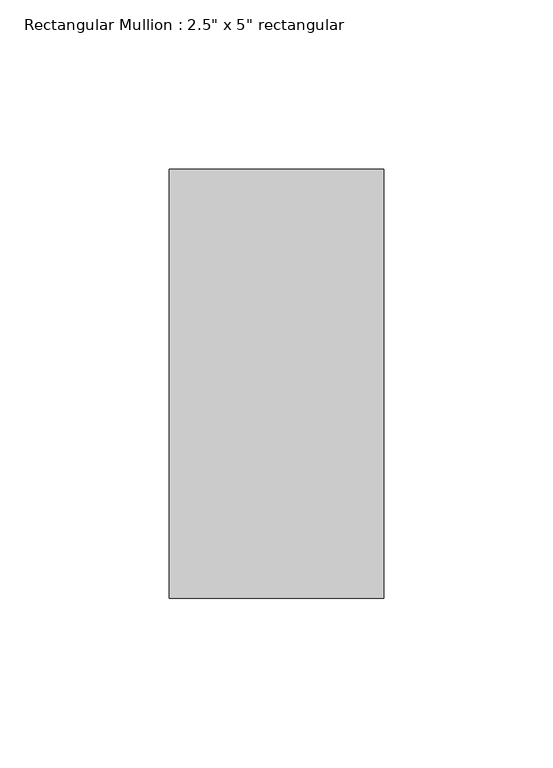
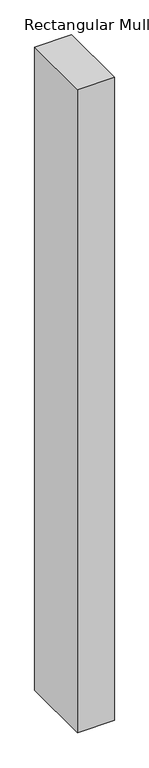
"""IFC4 building model written with IfcOpenShell, lengths in millimetres: member geometry."""

from ifc_helpers import new_model, si_unit, frame, origin, place, context, project, spatial, polyline, outline, extrude, source, transform, mapped, element, save


def member_476d3acb(model_context):
    return source(origin(), model_context, "Body", "SweptSolid", [
        extrude(outline(polyline([(0.0, 63.5), (0.0, -63.5), (-63.5, -63.5), (-63.5, 63.5), (0.0, 63.5)])), frame((0.0, 0.0, -1168.4), z_axis=(0.0, 0.0, 1.0), x_axis=(1.0, 0.0, 0.0)), (0.0, 0.0, 1.0), 1168.4),
    ])


if __name__ == "__main__":
    model = new_model("IFC4")
    model_context = context("Model", 3, world=origin())
    ifc_project = project(units=[si_unit("LENGTHUNIT", "METRE", prefix="MILLI")], contexts=[model_context])
    site = spatial("IfcSite", under=ifc_project)
    building = spatial("IfcBuilding", under=site)
    placement = place(None, origin())
    member_shape = member_476d3acb(model_context)
    element("IfcMember", 1, ObjectType="Rectangular Mullion : 2.5\" x 5\" rectangular", at=placement, inside=building, context=model_context, shape_type="MappedRepresentation", body=[
        mapped(member_shape, transform((0.0, 0.0, 0.0), x_axis=(1.0, 0.0, 0.0), y_axis=(0.0, 1.0, 0.0), z_axis=(0.0, 0.0, 1.0))),
    ])
    save(model, "model.ifc")

# Revit data of these elements
# Type "Rectangular Mullion : 2.5\" x 5\" rectangular"
#   built-in parameter 1007304 = 0.416667 (stored number, unit not read)
#   built-in parameter 1007301 = 0.104167 (stored number, unit not read)
#   built-in parameter 1007300 = 0.104167 (stored number, unit not read)
# Element 1 (IfcMember, "Rectangular Mullion : 2.5\" x 5\" rectangular")
#   Materials on its faces: "Aluminum"
# Materials
#   "Aluminum": class "Metal", colour RGB 247 247 247, transparency 0, Description = "Aluminum 6061", Cost = 0
